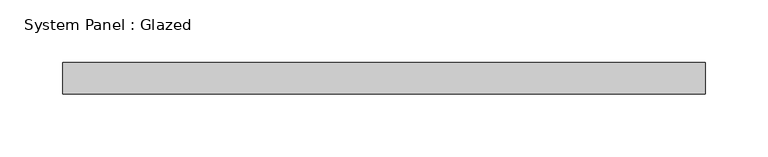
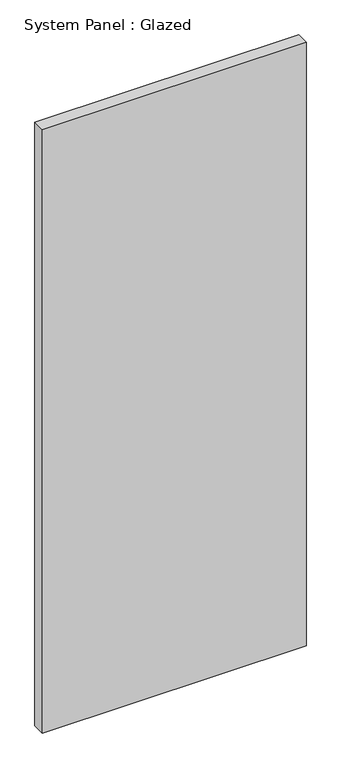
"""IFC4 building model written with IfcOpenShell, lengths in millimetres: plate geometry, System Panel : Glazed."""

from ifc_helpers import new_model, si_unit, origin, origin_with_axes, place, context, project, spatial, polyline, outline, extrude, source, transform, mapped, element, save


def system_panel_glazed_df5e78e0(model_context):
    return source(origin(), model_context, "Body", "SweptSolid", [
        extrude(outline(polyline([(257.175, 19.05), (-257.175, 19.05), (-257.175, 44.45), (257.175, 44.45), (257.175, 19.05)])), origin_with_axes(), (0.0, 0.0, 1.0), 1244.6),
    ])


if __name__ == "__main__":
    model = new_model("IFC4")
    model_context = context("Model", 3, world=origin())
    ifc_project = project(units=[si_unit("LENGTHUNIT", "METRE", prefix="MILLI")], contexts=[model_context])
    site = spatial("IfcSite", under=ifc_project)
    building = spatial("IfcBuilding", under=site)
    placement = place(None, origin())
    system_panel_glazed_shape = system_panel_glazed_df5e78e0(model_context)
    element("IfcPlate", 1, ObjectType="System Panel : Glazed", at=placement, inside=building, context=model_context, shape_type="MappedRepresentation", body=[
        mapped(system_panel_glazed_shape, transform((0.0, 0.0, 0.0), x_axis=(1.0, 0.0, 0.0), y_axis=(0.0, 1.0, 0.0), z_axis=(0.0, 0.0, 1.0))),
    ])
    save(model, "model.ifc")

# Revit data of these elements
# Type "System Panel : Glazed"
#   Construction Type Id = "GSP4R"
#   Analytic Construction = "1/8 in Pilkington single glazing"
#   Visual Light Transmittance = 0.9
#   Solar Heat Gain Coefficient = 0.86
#   Heat Transfer Coefficient (U) = 1.18115 BTU/(h·ft²·°F)
#   Define Thermal Properties by = 1
# Element 1 (IfcPlate, "System Panel : Glazed")
#   Materials on its faces: "Glass"
# Materials
#   "Glass": class "Glass", colour RGB 0 128 192, transparency 0.75, Description = "Soda Lime Glass", Cost = 0
